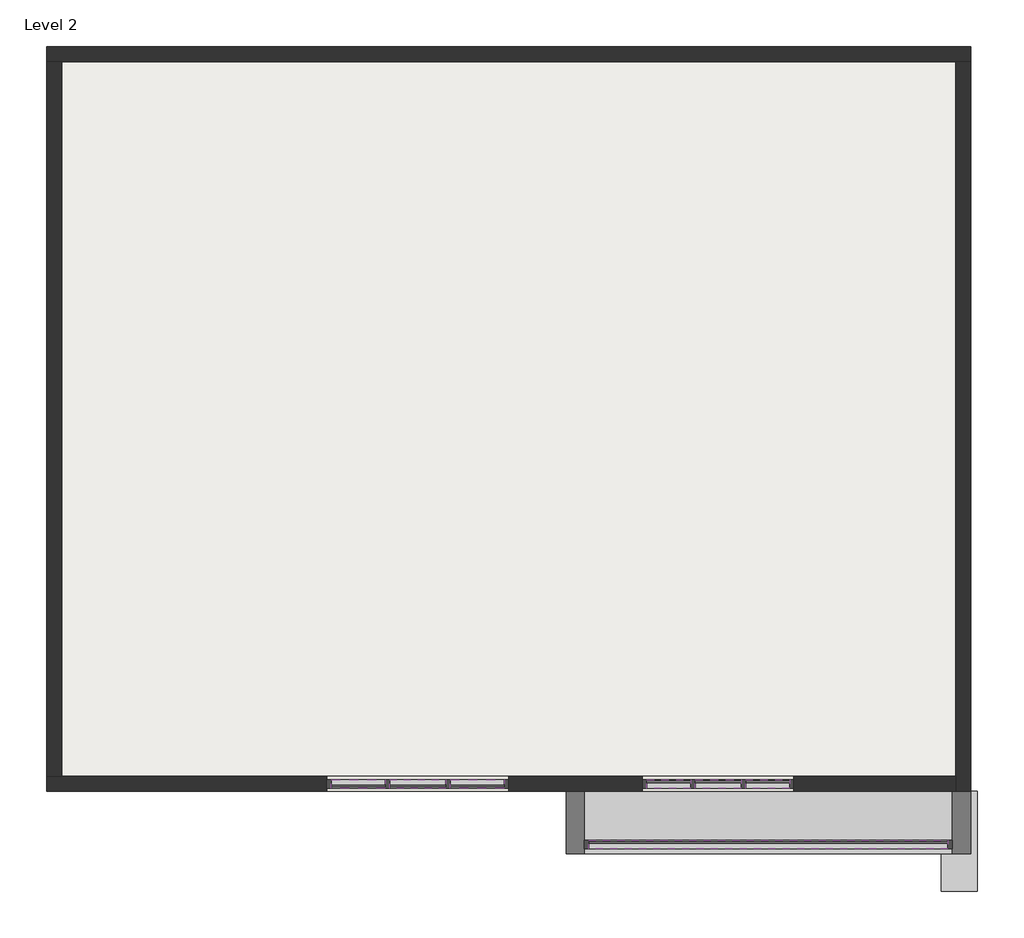
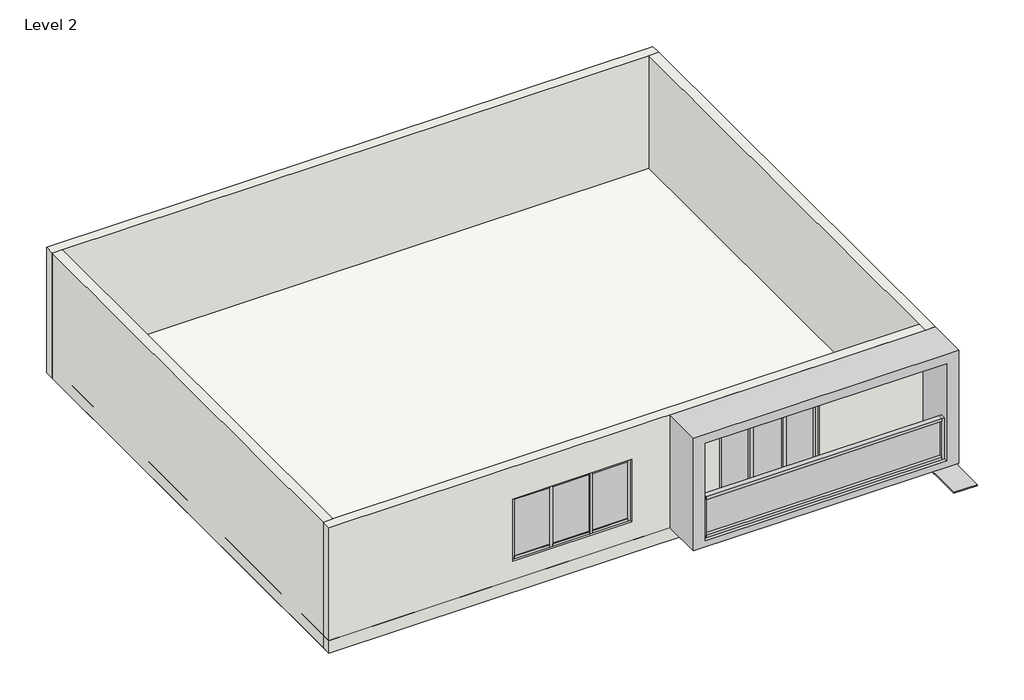
# One storey: 24 members, 7 plates, 4 walls, 2 proxies, 1 roof.
"""IFC4 building model written with IfcOpenShell, lengths in millimetres."""

from ifc_helpers import new_model, si_unit, frame, origin, place, context, project, spatial, polyline, outline, extrude, faceted_brep, transform, mapped, element, save
from components import generic_models_2_generic_models_2_26ab94c5, generic_models_5_generic_models_5_ba4ed622, member_c33c434a, member_d2e7e466, member_c17f1be2, member_c224591e, member_a31ba1dd, member_b955a9e9, member_0a963142, member_6a1115f2, member_769db2f1, member_ca7a94d5, system_panel_glazed_c96ed355, system_panel_glazed_3a3afa19, system_panel_glazed_903d0225, system_panel_glazed_30f93ba9, system_panel_glazed_62b5ff2e

model = new_model("IFC4")

# Units and contexts
model_context = context("Model", 3, world=origin())
ifc_project = project(units=[si_unit("LENGTHUNIT", "METRE", prefix="MILLI")], contexts=[model_context])

# Site, building, storey
site = spatial("IfcSite", under=ifc_project)
building = spatial("IfcBuilding", under=site)
storey = spatial("IfcBuildingStorey", under=building, Name="Level 2", Elevation=3048.0)

# Proxies
placement = place(None, origin())
generic_models_2_generic_models_2_shape = generic_models_2_generic_models_2_26ab94c5(model_context)
element("IfcBuildingElementProxy", 1, Name="Generic Models 2 : Generic Models 2", ObjectType="Generic Models 2 : Generic Models 2", at=placement, inside=storey, context=model_context, shape_type="MappedRepresentation", body=[
    mapped(generic_models_2_generic_models_2_shape, transform((0.0, 0.0, 0.0), x_axis=(1.0, 0.0, 0.0), y_axis=(0.0, 1.0, 0.0), z_axis=(0.0, 0.0, 1.0))),
])
generic_models_5_generic_models_5_shape = generic_models_5_generic_models_5_ba4ed622(model_context)
element("IfcBuildingElementProxy", 2, Name="Generic Models 5 : Generic Models 5", ObjectType="Generic Models 5 : Generic Models 5", at=placement, inside=storey, context=model_context, shape_type="MappedRepresentation", body=[
    mapped(generic_models_5_generic_models_5_shape, transform((0.0, 0.0, 0.0), x_axis=(1.0, 0.0, 0.0), y_axis=(0.0, 1.0, 0.0), z_axis=(0.0, 0.0, 1.0))),
])

# Members
member_shape = member_c33c434a(model_context)
element("IfcMember", 3, ObjectType="Rectangular Mullion : 2.5\" x 5\" rectangular", at=placement, inside=storey, context=model_context, shape_type="MappedRepresentation", body=[
    mapped(member_shape, transform((-8801.0331929, -10172.1592534, 5871.6595085), x_axis=(0.0, 0.0, 1.0), y_axis=(0.0, -1.0, 0.0), z_axis=(1.0, 0.0, 0.0))),
])
element("IfcMember", 4, ObjectType="Rectangular Mullion : 2.5\" x 5\" rectangular", at=placement, inside=storey, context=model_context, shape_type="MappedRepresentation", body=[
    mapped(member_shape, transform((-7308.7831929, -10172.1592534, 5871.6595085), x_axis=(0.0, 0.0, 1.0), y_axis=(0.0, -1.0, 0.0), z_axis=(1.0, 0.0, 0.0))),
])
element("IfcMember", 5, ObjectType="Rectangular Mullion : 2.5\" x 5\" rectangular", at=placement, inside=storey, context=model_context, shape_type="MappedRepresentation", body=[
    mapped(member_shape, transform((-7975.5331929, -10172.1592534, 3507.0931812), x_axis=(0.0, 0.0, -1.0), y_axis=(0.0, -1.0, 0.0), z_axis=(-1.0, 0.0, 0.0))),
])
element("IfcMember", 6, ObjectType="Rectangular Mullion : 2.5\" x 5\" rectangular", at=placement, inside=storey, context=model_context, shape_type="MappedRepresentation", body=[
    mapped(member_shape, transform((-9467.7831929, -10172.1592534, 3507.0931812), x_axis=(0.0, 0.0, -1.0), y_axis=(0.0, -1.0, 0.0), z_axis=(-1.0, 0.0, 0.0))),
])
member_2_shape = member_d2e7e466(model_context)
element("IfcMember", 7, ObjectType="Rectangular Mullion : 2.5\" x 5\" rectangular", at=placement, inside=storey, context=model_context, shape_type="MappedRepresentation", body=[
    mapped(member_2_shape, transform((-13347.6331929, -10172.1592534, 5313.3697962), x_axis=(0.0, 0.0, 1.0), y_axis=(0.0, 1.0, 0.0), z_axis=(-1.0, 0.0, 0.0))),
])
member_3_shape = member_c17f1be2(model_context)
element("IfcMember", 8, ObjectType="Rectangular Mullion : 2.5\" x 5\" rectangular", at=placement, inside=storey, context=model_context, shape_type="MappedRepresentation", body=[
    mapped(member_3_shape, transform((-12433.2331929, -10172.1592534, 5313.3697962), x_axis=(0.0, 0.0, 1.0), y_axis=(0.0, 1.0, 0.0), z_axis=(-1.0, 0.0, 0.0))),
])
element("IfcMember", 9, ObjectType="Rectangular Mullion : 2.5\" x 5\" rectangular", at=placement, inside=storey, context=model_context, shape_type="MappedRepresentation", body=[
    mapped(member_3_shape, transform((-14230.2831929, -10172.1592534, 5313.3697962), x_axis=(0.0, 0.0, 1.0), y_axis=(0.0, 1.0, 0.0), z_axis=(-1.0, 0.0, 0.0))),
])
member_4_shape = member_c224591e(model_context)
element("IfcMember", 10, ObjectType="Rectangular Mullion : 2.5\" x 5\" rectangular", at=placement, inside=storey, context=model_context, shape_type="MappedRepresentation", body=[
    mapped(member_4_shape, transform((-13379.3831929, -10172.1592534, 3799.5834003), x_axis=(-1.0, 0.0, 0.0), y_axis=(0.0, 1.0, 0.0), z_axis=(0.0, 0.0, -1.0))),
])
element("IfcMember", 11, ObjectType="Rectangular Mullion : 2.5\" x 5\" rectangular", at=placement, inside=storey, context=model_context, shape_type="MappedRepresentation", body=[
    mapped(member_4_shape, transform((-12464.9831929, -10172.1592534, 3799.5834003), x_axis=(-1.0, 0.0, 0.0), y_axis=(0.0, 1.0, 0.0), z_axis=(0.0, 0.0, -1.0))),
])
element("IfcMember", 12, ObjectType="Rectangular Mullion : 2.5\" x 5\" rectangular", at=placement, inside=storey, context=model_context, shape_type="MappedRepresentation", body=[
    mapped(member_2_shape, transform((-12496.7331929, -10172.1592534, 3799.5834003), x_axis=(0.0, 0.0, -1.0), y_axis=(0.0, 1.0, 0.0), z_axis=(1.0, 0.0, 0.0))),
])
element("IfcMember", 13, ObjectType="Rectangular Mullion : 2.5\" x 5\" rectangular", at=placement, inside=storey, context=model_context, shape_type="MappedRepresentation", body=[
    mapped(member_3_shape, transform((-13411.1331929, -10172.1592534, 3799.5834003), x_axis=(0.0, 0.0, -1.0), y_axis=(0.0, 1.0, 0.0), z_axis=(1.0, 0.0, 0.0))),
])
element("IfcMember", 14, ObjectType="Rectangular Mullion : 2.5\" x 5\" rectangular", at=placement, inside=storey, context=model_context, shape_type="MappedRepresentation", body=[
    mapped(member_3_shape, transform((-11614.0831929, -10172.1592534, 3799.5834003), x_axis=(0.0, 0.0, -1.0), y_axis=(0.0, 1.0, 0.0), z_axis=(1.0, 0.0, 0.0))),
])
member_5_shape = member_a31ba1dd(model_context)
element("IfcMember", 15, ObjectType="Rectangular Mullion : 2.5\" x 5\" rectangular", at=placement, inside=storey, context=model_context, shape_type="MappedRepresentation", body=[
    mapped(member_5_shape, transform((-14293.7831929, -10172.1592534, 3799.5834003), x_axis=(-1.0, 0.0, 0.0), y_axis=(0.0, 1.0, 0.0), z_axis=(0.0, 0.0, -1.0))),
])
element("IfcMember", 16, ObjectType="Rectangular Mullion : 2.5\" x 5\" rectangular", at=placement, inside=storey, context=model_context, shape_type="MappedRepresentation", body=[
    mapped(member_5_shape, transform((-11550.5831929, -10172.1592534, 5313.3697962), x_axis=(1.0, 0.0, 0.0), y_axis=(0.0, 1.0, 0.0), z_axis=(0.0, 0.0, 1.0))),
])
member_6_shape = member_b955a9e9(model_context)
element("IfcMember", 17, ObjectType="Rectangular Mullion : 2.5\" x 5\" rectangular", at=placement, inside=storey, context=model_context, shape_type="MappedRepresentation", body=[
    mapped(member_6_shape, transform((-8039.0331929, -10172.1592534, 5871.6595085), x_axis=(0.0, 0.0, 1.0), y_axis=(0.0, -1.0, 0.0), z_axis=(1.0, 0.0, 0.0))),
])
member_7_shape = member_0a963142(model_context)
element("IfcMember", 18, ObjectType="Rectangular Mullion : 2.5\" x 5\" rectangular", at=placement, inside=storey, context=model_context, shape_type="MappedRepresentation", body=[
    mapped(member_7_shape, transform((-8769.2831929, -10172.1592534, 3507.0931812), x_axis=(1.0, 0.0, 0.0), y_axis=(0.0, -1.0, 0.0), z_axis=(0.0, 0.0, -1.0))),
])
element("IfcMember", 19, ObjectType="Rectangular Mullion : 2.5\" x 5\" rectangular", at=placement, inside=storey, context=model_context, shape_type="MappedRepresentation", body=[
    mapped(member_7_shape, transform((-8007.2831929, -10172.1592534, 3507.0931812), x_axis=(1.0, 0.0, 0.0), y_axis=(0.0, -1.0, 0.0), z_axis=(0.0, 0.0, -1.0))),
])
element("IfcMember", 20, ObjectType="Rectangular Mullion : 2.5\" x 5\" rectangular", at=placement, inside=storey, context=model_context, shape_type="MappedRepresentation", body=[
    mapped(member_6_shape, transform((-8737.5331929, -10172.1592534, 3507.0931812), x_axis=(0.0, 0.0, -1.0), y_axis=(0.0, -1.0, 0.0), z_axis=(-1.0, 0.0, 0.0))),
])
member_8_shape = member_6a1115f2(model_context)
element("IfcMember", 21, ObjectType="Rectangular Mullion : 2.5\" x 5\" rectangular", at=placement, inside=storey, context=model_context, shape_type="MappedRepresentation", body=[
    mapped(member_8_shape, transform((-9531.2831929, -10172.1592534, 5871.6595085), x_axis=(-1.0, 0.0, 0.0), y_axis=(0.0, -1.0, 0.0), z_axis=(0.0, 0.0, 1.0))),
])
element("IfcMember", 22, ObjectType="Rectangular Mullion : 2.5\" x 5\" rectangular", at=placement, inside=storey, context=model_context, shape_type="MappedRepresentation", body=[
    mapped(member_8_shape, transform((-7245.2831929, -10172.1592534, 3507.0931812), x_axis=(1.0, 0.0, 0.0), y_axis=(0.0, -1.0, 0.0), z_axis=(0.0, 0.0, -1.0))),
])
member_9_shape = member_769db2f1(model_context)
element("IfcMember", 23, ObjectType="Rectangular Mullion : 2.5\" x 5\" rectangular", at=placement, inside=storey, context=model_context, shape_type="MappedRepresentation", body=[
    mapped(member_9_shape, transform((-10407.5831929, -11086.5592534, 4505.0543952), x_axis=(-1.0, 0.0, 0.0), y_axis=(0.0, -1.0, 0.0), z_axis=(0.0, 0.0, 1.0))),
])
member_10_shape = member_ca7a94d5(model_context)
element("IfcMember", 24, ObjectType="Rectangular Mullion : 2.5\" x 5\" rectangular", at=placement, inside=storey, context=model_context, shape_type="MappedRepresentation", body=[
    mapped(member_10_shape, transform((-4921.1831929, -11086.5592534, 4505.0543952), x_axis=(0.0, 0.0, 1.0), y_axis=(0.0, -1.0, 0.0), z_axis=(1.0, 0.0, 0.0))),
])
element("IfcMember", 25, ObjectType="Rectangular Mullion : 2.5\" x 5\" rectangular", at=placement, inside=storey, context=model_context, shape_type="MappedRepresentation", body=[
    mapped(member_10_shape, transform((-10344.0831929, -11086.5592534, 3507.0931812), x_axis=(0.0, 0.0, -1.0), y_axis=(0.0, -1.0, 0.0), z_axis=(-1.0, 0.0, 0.0))),
])
element("IfcMember", 26, ObjectType="Rectangular Mullion : 2.5\" x 5\" rectangular", at=placement, inside=storey, context=model_context, shape_type="MappedRepresentation", body=[
    mapped(member_9_shape, transform((-4857.6831929, -11086.5592534, 3507.0931812), x_axis=(1.0, 0.0, 0.0), y_axis=(0.0, -1.0, 0.0), z_axis=(0.0, 0.0, -1.0))),
])

# Plates
system_panel_glazed_shape = system_panel_glazed_c96ed355(model_context)
element("IfcPlate", 27, ObjectType="System Panel : Glazed", at=placement, inside=storey, context=model_context, shape_type="MappedRepresentation", body=[
    mapped(system_panel_glazed_shape, transform((-12023.6581929, -10172.1592534, 3863.0834003), x_axis=(-1.0, 0.0, 0.0), y_axis=(0.0, -1.0, 0.0), z_axis=(0.0, 0.0, 1.0))),
])
element("IfcPlate", 28, ObjectType="System Panel : Glazed", at=placement, inside=storey, context=model_context, shape_type="MappedRepresentation", body=[
    mapped(system_panel_glazed_shape, transform((-13820.7081929, -10172.1592534, 3863.0834003), x_axis=(-1.0, 0.0, 0.0), y_axis=(0.0, -1.0, 0.0), z_axis=(0.0, 0.0, 1.0))),
])
system_panel_glazed_2_shape = system_panel_glazed_3a3afa19(model_context)
element("IfcPlate", 29, ObjectType="System Panel : Glazed", at=placement, inside=storey, context=model_context, shape_type="MappedRepresentation", body=[
    mapped(system_panel_glazed_2_shape, transform((-12922.1831929, -10172.1592534, 3863.0834003), x_axis=(-1.0, 0.0, 0.0), y_axis=(0.0, -1.0, 0.0), z_axis=(0.0, 0.0, 1.0))),
])
system_panel_glazed_3_shape = system_panel_glazed_903d0225(model_context)
element("IfcPlate", 30, ObjectType="System Panel : Glazed", at=placement, inside=storey, context=model_context, shape_type="MappedRepresentation", body=[
    mapped(system_panel_glazed_3_shape, transform((-9134.4081929, -10172.1592534, 3570.5931812), x_axis=(1.0, 0.0, 0.0), y_axis=(0.0, 1.0, 0.0), z_axis=(0.0, 0.0, 1.0))),
])
element("IfcPlate", 31, ObjectType="System Panel : Glazed", at=placement, inside=storey, context=model_context, shape_type="MappedRepresentation", body=[
    mapped(system_panel_glazed_3_shape, transform((-7642.1581929, -10172.1592534, 3570.5931812), x_axis=(1.0, 0.0, 0.0), y_axis=(0.0, 1.0, 0.0), z_axis=(0.0, 0.0, 1.0))),
])
system_panel_glazed_4_shape = system_panel_glazed_30f93ba9(model_context)
element("IfcPlate", 32, ObjectType="System Panel : Glazed", at=placement, inside=storey, context=model_context, shape_type="MappedRepresentation", body=[
    mapped(system_panel_glazed_4_shape, transform((-8388.2831929, -10172.1592534, 3570.5931812), x_axis=(1.0, 0.0, 0.0), y_axis=(0.0, 1.0, 0.0), z_axis=(0.0, 0.0, 1.0))),
])
system_panel_glazed_5_shape = system_panel_glazed_62b5ff2e(model_context)
element("IfcPlate", 33, ObjectType="System Panel : Glazed", at=placement, inside=storey, context=model_context, shape_type="MappedRepresentation", body=[
    mapped(system_panel_glazed_5_shape, transform((-7632.6331929, -11086.5592534, 3570.5931812), x_axis=(1.0, 0.0, 0.0), y_axis=(0.0, 1.0, 0.0), z_axis=(0.0, 0.0, 1.0))),
])

# Roof
element("IfcRoof", 34, ObjectType="Generic - 12\"", at=placement, inside=storey, context=model_context, shape_type="SweptSolid", body=[
    extrude(outline(polyline([(-18522.8831929, 953.0407466), (-4578.2831929, 953.0407466), (-4578.2831929, -10286.4592534), (-18522.8831929, -10286.4592534), (-18522.8831929, 953.0407466)])), frame((0.0, 0.0, 3048.0), z_axis=(0.0, 0.0, 1.0), x_axis=(1.0, 0.0, 0.0)), (0.0, 0.0, 1.0), 304.8),
])

# Walls
element("IfcWall", 35, ObjectType="9\"", at=placement, inside=storey, context=model_context, shape_type="Brep", body=[
    faceted_brep([(-18522.8831929, 724.4407466, 3048.0), (-18294.2831929, 724.4407466, 3048.0), (-4806.8831929, 724.4407466, 3048.0), (-4578.2831929, 724.4407466, 3048.0), (-4578.2831929, 724.4407466, 6096.0), (-4806.8831929, 724.4407466, 6096.0), (-18294.2831929, 724.4407466, 6096.0), (-18522.8831929, 724.4407466, 6096.0), (-18522.8831929, 953.0407466, 3048.0), (-18522.8831929, 953.0407466, 6096.0), (-4578.2831929, 953.0407466, 6096.0), (-4578.2831929, 953.0407466, 3048.0)], [[[0, 1, 2, 3, 4, 5, 6, 7]], [[8, 9, 10, 11]], [[3, 2, 1, 0, 8, 11]], [[7, 6, 5, 4, 10, 9]], [[4, 3, 11, 10]], [[0, 7, 9, 8]]]),
])
element("IfcWall", 36, ObjectType="9\"", at=placement, inside=storey, context=model_context, shape_type="Brep", body=[
    faceted_brep([(-4806.8831929, 724.4407466, 3048.0), (-4806.8831929, -10057.8592534, 3048.0), (-4806.8831929, -10286.4592534, 3048.0), (-4806.8831929, -10286.4592534, 6096.0), (-4806.8831929, -10057.8592534, 6096.0), (-4806.8831929, 724.4407466, 6096.0), (-4578.2831929, 724.4407466, 3048.0), (-4578.2831929, 724.4407466, 6096.0), (-4578.2831929, -10286.4592534, 6096.0), (-4578.2831929, -10286.4592534, 3048.0)], [[[0, 1, 2, 3, 4, 5]], [[6, 7, 8, 9]], [[2, 1, 0, 6, 9]], [[5, 4, 3, 8, 7]], [[0, 5, 7, 6]], [[3, 2, 9, 8]]]),
])
element("IfcWall", 37, ObjectType="9\"", at=placement, inside=storey, context=model_context, shape_type="Brep", body=[
    faceted_brep([(-4806.8831929, -10057.8592534, 3048.0), (-18294.2831929, -10057.8592534, 3048.0), (-18522.8831929, -10057.8592534, 3048.0), (-18522.8831929, -10057.8592534, 6096.0), (-18294.2831929, -10057.8592534, 6096.0), (-4806.8831929, -10057.8592534, 6096.0), (-9531.2831929, -10057.8592534, 5871.6595085), (-9531.2831929, -10057.8592534, 3507.0931812), (-7245.2831929, -10057.8592534, 3507.0931812), (-7245.2831929, -10057.8592534, 5871.6595085), (-11550.5831929, -10057.8592534, 3799.5834003), (-11550.5831929, -10057.8592534, 5313.3697962), (-14293.7831929, -10057.8592534, 5313.3697962), (-14293.7831929, -10057.8592534, 3799.5834003), (-18522.8831929, -10286.4592534, 3048.0), (-4806.8831929, -10286.4592534, 3048.0), (-4806.8831929, -10286.4592534, 6096.0), (-18522.8831929, -10286.4592534, 6096.0), (-9531.2831929, -10286.4592534, 3507.0931812), (-9531.2831929, -10286.4592534, 5871.6595085), (-7245.2831929, -10286.4592534, 5871.6595085), (-7245.2831929, -10286.4592534, 3507.0931812), (-11550.5831929, -10286.4592534, 5313.3697962), (-11550.5831929, -10286.4592534, 3799.5834003), (-14293.7831929, -10286.4592534, 3799.5834003), (-14293.7831929, -10286.4592534, 5313.3697962)], [[[0, 1, 2, 3, 4, 5], [6, 7, 8, 9], [10, 11, 12, 13]], [[14, 15, 16, 17], [18, 19, 20, 21], [22, 23, 24, 25]], [[2, 1, 0, 15, 14]], [[5, 4, 3, 17, 16]], [[0, 5, 16, 15]], [[3, 2, 14, 17]], [[6, 19, 18, 7]], [[19, 6, 9, 20]], [[20, 9, 8, 21]], [[7, 18, 21, 8]], [[10, 23, 22, 11]], [[11, 22, 25, 12]], [[12, 25, 24, 13]], [[23, 10, 13, 24]]]),
])
element("IfcWall", 38, ObjectType="9\"", at=placement, inside=storey, context=model_context, shape_type="SweptSolid", body=[
    extrude(outline(polyline([(-18294.2831929, 724.4407466), (-18294.2831929, -10057.8592534), (-18522.8831929, -10057.8592534), (-18522.8831929, 724.4407466), (-18294.2831929, 724.4407466)])), frame((0.0, 0.0, 3048.0), z_axis=(0.0, 0.0, 1.0), x_axis=(1.0, 0.0, 0.0)), (0.0, 0.0, 1.0), 3048.0),
])

save(model, "model.ifc")

# Revit data of these elements
# Type "Rectangular Mullion : 2.5\" x 5\" rectangular"
#   built-in parameter 1007304 = 0.416667 (stored number, unit not read)
#   built-in parameter 1007301 = 0.104167 (stored number, unit not read)
#   built-in parameter 1007300 = 0.104167 (stored number, unit not read)
# Type "System Panel : Glazed"
#   Construction Type Id = "GSP4R"
#   Analytic Construction = "1/8 in Pilkington single glazing"
#   Visual Light Transmittance = 0.9
#   Solar Heat Gain Coefficient = 0.86
#   Heat Transfer Coefficient (U) = 1.18115 BTU/(h·ft²·°F)
#   Define Thermal Properties by = 1
# Type "Generic - 12\""
#   Assembly Code = "B1020"
#   Layers, outside or top first: 1' - 0" no material (function 1)
# Type "9\""
#   Assembly Code = "B2010"
#   Layers, outside or top first: 0' - 9" no material (function 1)
# Element 1 (IfcBuildingElementProxy, "Generic Models 2 : Generic Models 2")
#   Phase Created = New Construction
# Element 2 (IfcBuildingElementProxy, "Generic Models 5 : Generic Models 5")
#   Phase Created = New Construction
# Elements 3, 4, 5, 6, 7, 8, 9, 10, 11, 12, 13, 14, 15, 16, 17, 18, 19, 20, 21, 22, 23, 24, 25, 26 (IfcMember, "Rectangular Mullion : 2.5\" x 5\" rectangular")
#   Phase Created = New Construction
#   Materials on its faces: "Aluminum"
# Elements 27, 28, 29, 30, 31, 32, 33 (IfcPlate, "System Panel : Glazed")
#   Phase Created = New Construction
#   Materials on its faces: "Glass"
# Element 34 (IfcRoof, "Generic - 12\"")
#   built-in parameter 1001705 = 11 (stored number, unit not read)
#   built-in parameter 1001710 = 33615
#   Phase Created = New Construction
#   Materials on its faces: "Default Roof"
# Elements 35, 36, 37, 38 (IfcWall, "9\"")
#   Top Offset = 0' - 0"
#   Base Offset = 0' - 0"
#   Unconnected Height = 10' - 0"
#   wall height = 10' - 0"
#   Phase Created = New Construction
#   Base Constraint = Level 2
#   Materials on its faces: "Default Wall"
# Materials
#   "Aluminum": class "Metal", colour RGB 247 247 247, transparency 0, Description = "Aluminum 6061", Cost = 0
#   "Glass": class "Glass", colour RGB 0 128 192, transparency 0.75, Description = "Soda Lime Glass", Cost = 0
#   "Default Roof": colour RGB 88 101 114, transparency 0, Cost = 0
#   "Default Wall": colour RGB 128 128 128, transparency 0, Cost = 0
